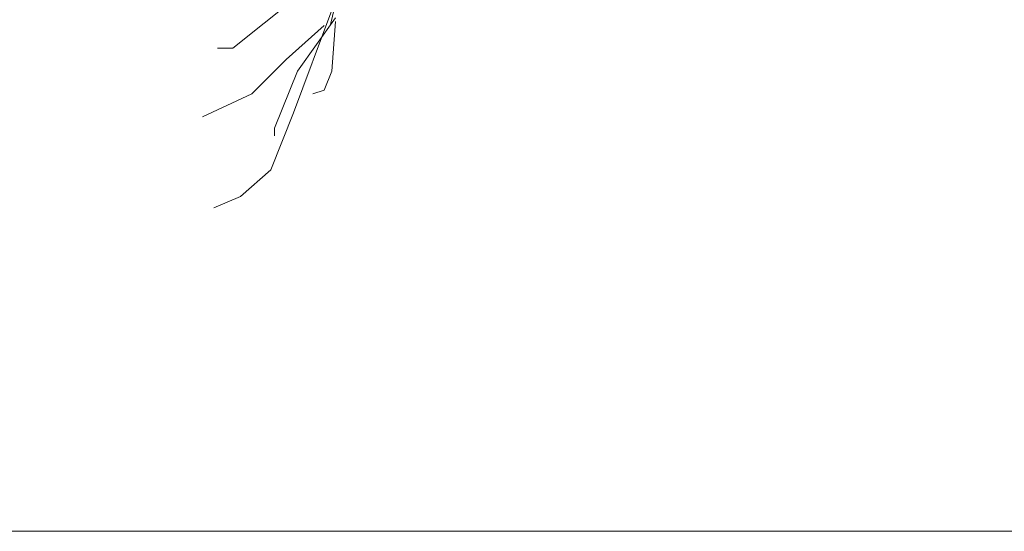
# Model space of a CAD drawing. Units: millimetres. Extents: x 595116 to 630915, y 909473 to 920225.
# Tile 97 of 134: x 629805.265 to 629812.676, y 919160.917 to 919164.766. Entities that reach past the tile are written whole.
import ezdxf

# ---------------------------------------------------------------- set-up
doc = ezdxf.new("R2010")
doc.units = ezdxf.units.MM
doc.layers.add('L-PLNT', color=85, linetype='Continuous', lineweight=13)

# ---------------------------------------------------------------- blocks, each defined once
blk = doc.blocks.new('A$C4FB75ABC')
for p, q in [((3.2869, 0.4726), (3.0962, 0.3201)), ((3.3124, 0.4531), (3.2923, 0.3674)), ((3.2945, 0.3964), (3.2182, 0.1906)), ((3.3021, 0.3811), (3.2259, 0.2744)), ((3.2793, 0.3659), (3.203, 0.2973)), ((3.3021, 0.3735), (3.2945, 0.2744)), ((3.0962, 0.3201), (3.0657, 0.3201)), ((3.203, 0.2973), (3.1344, 0.2287)), ((3.2259, 0.2744), (3.1954, 0.1982)), ((3.2945, 0.2744), (3.2793, 0.2363)), ((3.1344, 0.2287), (3.0352, 0.1829)), ((3.2793, 0.2363), (3.2564, 0.2287)), ((3.1954, 0.1982), (3.1801, 0.1601)), ((3.2182, 0.1906), (3.1725, 0.0762)), ((3.1801, 0.1601), (3.1801, 0.1448)), ((3.1725, 0.0762), (3.1115, 0.0229)), ((3.1115, 0.0229), (3.0581, 0))]:
    blk.add_line(p, q)

msp = doc.modelspace()

# ---------------------------------------------------------------- linework, layer by layer
at = {"layer": 'L-PLNT'}
msp.add_line((629511.2737, 919160.9171), (629824.9514, 919160.9171), dxfattribs=at)

# ---------------------------------------------------------------- block references
at = {"layer": 'L-PLNT', "xscale": 3.753413438031968, "yscale": 3.753413438031968, "zscale": 3.753413438031968}
msp.add_blockref('A$C4FB75ABC', (629795.2477, 919163.3497), dxfattribs=at)

doc.saveas('drawing.dxf')
